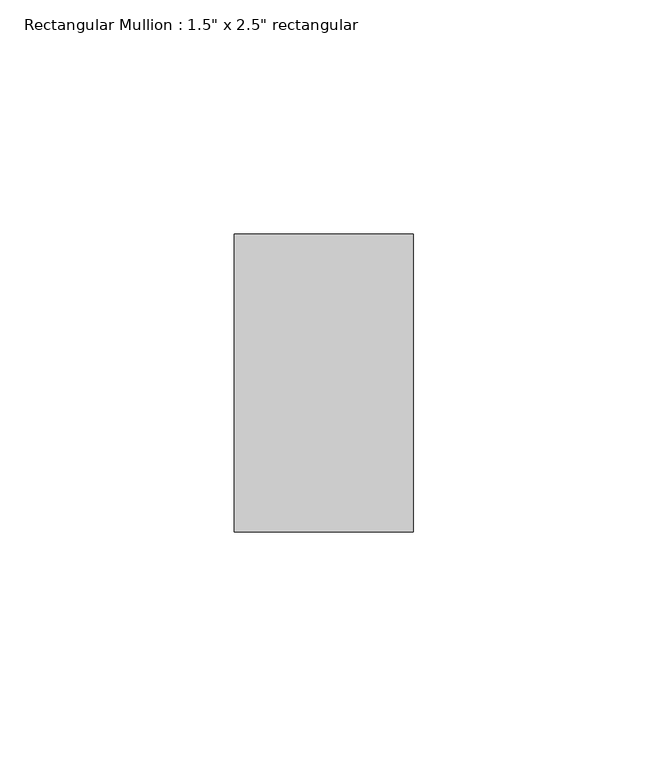
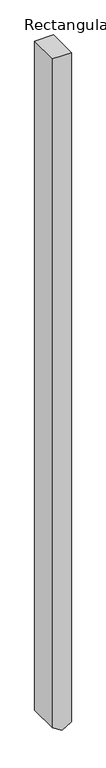
"""IFC4 building model written with IfcOpenShell, lengths in millimetres: member geometry."""

from ifc_helpers import new_model, si_unit, frame, origin, place, context, project, spatial, polyline, outline, extrude, source, transform, mapped, element, save


def member_3c184fc8(model_context):
    return source(origin(), model_context, "Body", "SweptSolid", [
        extrude(outline(polyline([(0.0, 19.05), (0.0, -19.05), (-1443.9853958, -19.05), (-1455.3076527, 0.0), (-1443.9853958, 19.05), (0.0, 19.05)])), frame((0.0, -31.75, 0.0), z_axis=(0.0, 1.0, 0.0), x_axis=(0.0, 0.0, 1.0)), (0.0, 0.0, 1.0), 63.5),
    ])


if __name__ == "__main__":
    model = new_model("IFC4")
    model_context = context("Model", 3, world=origin())
    ifc_project = project(units=[si_unit("LENGTHUNIT", "METRE", prefix="MILLI")], contexts=[model_context])
    site = spatial("IfcSite", under=ifc_project)
    building = spatial("IfcBuilding", under=site)
    placement = place(None, origin())
    member_shape = member_3c184fc8(model_context)
    element("IfcMember", 1, ObjectType="Rectangular Mullion : 1.5\" x 2.5\" rectangular", at=placement, inside=building, context=model_context, shape_type="MappedRepresentation", body=[
        mapped(member_shape, transform((0.0, 0.0, 0.0), x_axis=(1.0, 0.0, 0.0), y_axis=(0.0, 1.0, 0.0), z_axis=(0.0, 0.0, 1.0))),
    ])
    save(model, "model.ifc")

# Revit data of these elements
# Type "Rectangular Mullion : 1.5\" x 2.5\" rectangular"
#   built-in parameter 1007304 = 0.208333 (stored number, unit not read)
#   built-in parameter 1007301 = 0.0625 (stored number, unit not read)
#   built-in parameter 1007300 = 0.0625 (stored number, unit not read)
